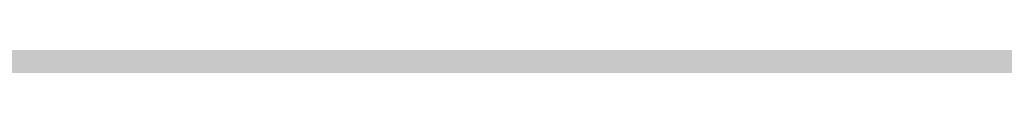
# Model space of a CAD drawing. Units: millimetres. Extents: x 0 to 2267, y 0 to 1823.
# Tile 98 of 256: x 1600.369 to 1605.705, y 1227.263 to 1227.331. Entities that reach past the tile are written whole.
import ezdxf

# ---------------------------------------------------------------- set-up
doc = ezdxf.new("R2010")
doc.units = ezdxf.units.MM
doc.header["$MEASUREMENT"] = 0
doc.layers.add('M-DIMS', color=2, linetype='Continuous', lineweight=25)
doc.layers.add('M-HATC', color=252, linetype='Continuous', lineweight=18)
doc.styles.get("Standard").update_dxf_attribs({"font": 'arial.ttf'})
doc.dimstyles.get("Standard").update_dxf_attribs({"dimtxt": 7, "dimasz": 4, "dimexe": 0.18, "dimexo": 0.0625, "dimgap": 0.09, "dimtad": 0, "dimdec": 0, "dimzin": 0, "dimdsep": 46, "dimtxsty": 'Standard', "dimcen": 0.09, "dimadec": 0, "dimazin": 0, "dimtfac": 1, "dimtdec": 0, "dimtofl": 0, "dimtmove": 0, "dimatfit": 3, "dimfxl": 1, "dimtolj": 1, "dimtzin": 0, "dimarcsym": 0})

# ---------------------------------------------------------------- blocks, each defined once
blk = doc.blocks.new('*D19')
at = {"layer": 'Defpoints', "color": 0, "transparency": 16777216}
for p in [(1605.3399, 1483.3044), (1445.5291, 1333.8851)]:
    blk.add_point(p, dxfattribs=at)
at = {"layer": 'M-DIMS', "color": 0, "lineweight": -2, "transparency": 16777216}
for p, q in [((1605.3399, 1483.2144), (1605.3399, 1483.3944)), ((1605.2499, 1483.3044), (1605.4299, 1483.3044)), ((1366.3244, 1259.8306), (1442.6072, 1331.1532))]:
    blk.add_line(p, q, dxfattribs=at)
at = {"layer": 'M-DIMS', "color": 0, "transparency": 16777216}
blk.add_solid([(1442.1519, 1331.6402), (1443.0625, 1330.6663), (1445.5291, 1333.8851)], dxfattribs=at)
at = {"layer": 'M-DIMS', "color": 0, "transparency": 16777216, "insert": (1349.6425, 1244.2335), "char_height": 7, "attachment_point": 5, "rotation": 43.0753}
blk.add_mtext('\\A1;2X R218.8', dxfattribs=at)

msp = doc.modelspace()

# ---------------------------------------------------------------- hatches: boundary and pattern name
at = {"layer": 'M-HATC'}
h = msp.add_hatch(color=256, dxfattribs=at)
h.dxf.hatch_style = 1
h.paths.add_polyline_path([(2055.771, 1603.062), (1381.0868, 1603.062), (1381.0868, 1598.062), (2055.771, 1598.062)])
h.paths.add_polyline_path([(2055.771, 1598.062), (1381.0868, 1598.062), (1381.0868, 1593.062), (2055.771, 1593.062)])
h.paths.add_polyline_path([(2051.3074, 1536.7609), (1385.5504, 1536.7609), (1385.5504, 1526.7609), (1387.5504, 1526.7609), (1388.5366, 1525.0528), (1385.3319, 1521.2335), (1385.3319, 1521.2226), (2050.2542, 1522.7491), (2048.3212, 1525.0528), (2049.3074, 1526.7609), (2051.3074, 1526.7609)])
edge = h.paths.add_edge_path()
edge.add_arc((1847.5345, 1379.1492), 135, 222.603061, 222.890851, ccw=False)
edge.add_line((1748.1663, 1287.7656), (1683.0921, 1287.7656))
edge.add_arc((1583.7239, 1379.1492), 135, 317.109149, 317.396939, ccw=False)
edge.add_arc((1678.9686, 1290.6707), 5, 222.8909, 317.1091, ccw=False)
edge.add_arc((1774.2133, 1379.1492), 135, 222.603061, 222.890851, ccw=False)
edge.add_line((1674.8451, 1287.7656), (1609.7709, 1287.7656))
edge.add_arc((1510.4027, 1379.1492), 135, 317.109149, 317.396939, ccw=False)
edge.add_arc((1605.6474, 1290.6707), 5, 222.8909, 317.1091, ccw=False)
edge.add_arc((1700.8921, 1379.1492), 135, 222.603061, 222.890851, ccw=False)
edge.add_line((1601.5239, 1287.7656), (1536.4497, 1287.7656))
edge.add_arc((1437.0815, 1379.1492), 135, 317.109149, 317.396939, ccw=False)
edge.add_arc((1532.3262, 1290.6707), 5, 222.8909, 317.1091, ccw=False)
edge.add_arc((1627.5709, 1379.1492), 135, 222.603061, 222.890851, ccw=False)
edge.add_line((1528.2027, 1287.7656), (1505.9289, 1287.7656))
edge.add_spline(control_points=[(1505.9289, 1287.7656), (1504.2622, 1287.7656), (1504.2622, 1282.7656), (1505.9289, 1282.7656)], knot_values=[0, 0, 0, 0, 5, 5, 5, 5], degree=3, periodic=0)
edge.add_line((1505.9289, 1282.7656), (1930.9289, 1282.7656))
edge.add_spline(control_points=[(1930.9289, 1282.7656), (1932.5956, 1282.7656), (1932.5956, 1287.7656), (1930.9289, 1287.7656)], knot_values=[0, 0, 0, 0, 5, 5, 5, 5], degree=3, periodic=0)
edge.add_line((1930.9289, 1287.7656), (1903.0557, 1287.7656))
edge.add_arc((1803.6875, 1379.1492), 135, 317.109149, 317.396939, ccw=False)
edge.add_arc((1898.9322, 1290.6707), 5, 222.8909, 317.1091, ccw=False)
edge.add_arc((1994.1769, 1379.1492), 135, 222.603061, 222.890851, ccw=False)
edge.add_line((1894.8087, 1287.7656), (1829.7345, 1287.7656))
edge.add_arc((1730.3663, 1379.1492), 135, 317.109149, 317.396939, ccw=False)
edge.add_arc((1825.611, 1290.6707), 5, 222.8909, 317.1091, ccw=False)
edge.add_arc((1920.8557, 1379.1492), 135, 222.603061, 222.890851, ccw=False)
edge.add_line((1821.4875, 1287.7656), (1756.4133, 1287.7656))
edge.add_arc((1657.0451, 1379.1492), 135, 317.109149, 317.396939, ccw=False)
edge.add_arc((1752.2898, 1290.6707), 5, 222.8909, 317.1091, ccw=False)
edge = h.paths.add_edge_path()
edge.add_spline(control_points=[(1843.4289, 1227.2475), (1845.0956, 1227.2475), (1845.0956, 1232.2475), (1843.4289, 1232.2475)], knot_values=[0, 0, 0, 0, 5, 5, 5, 5], degree=3, periodic=0)
edge.add_line((1843.4289, 1232.2475), (1593.4289, 1232.2475))
edge.add_spline(control_points=[(1593.4289, 1232.2475), (1591.7622, 1232.2475), (1591.7622, 1227.2475), (1593.4289, 1227.2475)], knot_values=[0, 0, 0, 0, 5, 5, 5, 5], degree=3, periodic=0)
edge.add_line((1593.4289, 1227.2475), (1843.4289, 1227.2475))
h.paths.add_polyline_path([(1905.9289, 1127.4171), (1530.9289, 1127.4171, 0.414214), (1520.9289, 1117.4171), (1530.9289, 1117.4171), (1915.9289, 1117.4171, 0.414214)])
edge = h.paths.add_edge_path()
edge.add_arc((1397.0858, 1498.4078), 12.7299, 90.78215, 190.87871, ccw=False)
edge.add_line((1396.912, 1511.1365), (1428.0097, 1511.3488))
edge.add_line((1428.0097, 1511.3488), (1433.0097, 1511.3488))
edge.add_line((1433.0097, 1511.3488), (1434.439, 1511.3488))
edge.add_arc((1419.474, 1498.0804), 20, 41.561, 74.08211)
edge.add_line((1424.9592, 1517.3135), (1399.9351, 1517.2561))
edge.add_spline(control_points=[(1399.9307, 1517.2561), (1399.884, 1517.2131), (1399.8328, 1517.1689), (1399.7774, 1517.1236)], knot_values=[11.567499, 11.567499, 11.567499, 11.567499, 11.814249, 11.814249, 11.814249, 11.814249], degree=3, periodic=0)
edge.add_spline(control_points=[(1399.6328, 1517.0099), (1399.5831, 1516.9721), (1399.5307, 1516.9338), (1399.4759, 1516.8947)], knot_values=[11.167718, 11.167718, 11.167718, 11.167718, 11.365188, 11.365188, 11.365188, 11.365188], degree=3, periodic=0)
edge.add_spline(control_points=[(1399.3398, 1516.8001), (1399.1514, 1516.6719), (1398.9384, 1516.5377), (1398.704, 1516.3994)], knot_values=[10.376405, 10.376405, 10.376405, 10.376405, 11.00994, 11.00994, 11.00994, 11.00994], degree=3, periodic=0)
edge.add_spline(control_points=[(1398.6572, 1516.3719), (1398.5789, 1516.326), (1398.4983, 1516.2797), (1398.4155, 1516.2331)], knot_values=[10.125175, 10.125175, 10.125175, 10.125175, 10.334406, 10.334406, 10.334406, 10.334406], degree=3, periodic=0)
edge.add_spline(control_points=[(1398.2642, 1516.1487), (1398.196, 1516.1111), (1398.1263, 1516.0732), (1398.0555, 1516.0351)], knot_values=[9.832246, 9.832246, 9.832246, 9.832246, 9.999658, 9.999658, 9.999658, 9.999658], degree=3, periodic=0)
edge.add_spline(control_points=[(1397.9987, 1516.0048), (1397.7312, 1515.8621), (1397.446, 1515.7171), (1397.1466, 1515.5714)], knot_values=[9.161808, 9.161808, 9.161808, 9.161808, 9.787769, 9.787769, 9.787769, 9.787769], degree=3, periodic=0)
edge.add_spline(control_points=[(1397.1466, 1515.5714), (1396.8418, 1515.423), (1396.5222, 1515.274), (1396.1914, 1515.1262)], knot_values=[8.524455, 8.524455, 8.524455, 8.524455, 9.161808, 9.161808, 9.161808, 9.161808], degree=3, periodic=0)
edge.add_spline(control_points=[(1396.0777, 1515.0756), (1395.9854, 1515.0348), (1395.8922, 1514.994), (1395.7983, 1514.9534)], knot_values=[8.275193, 8.275193, 8.275193, 8.275193, 8.451726, 8.451726, 8.451726, 8.451726], degree=3, periodic=0)
edge.add_spline(control_points=[(1395.6018, 1514.8691), (1395.4997, 1514.8257), (1395.3968, 1514.7824), (1395.2932, 1514.7394)], knot_values=[7.962917, 7.962917, 7.962917, 7.962917, 8.152764, 8.152764, 8.152764, 8.152764], degree=3, periodic=0)
edge.add_spline(control_points=[(1395.2116, 1514.7057), (1394.8278, 1514.5475), (1394.4345, 1514.3929), (1394.0364, 1514.2442)], knot_values=[7.21254, 7.21254, 7.21254, 7.21254, 7.913148, 7.913148, 7.913148, 7.913148], degree=3, periodic=0)
edge.add_spline(control_points=[(1394.0364, 1514.2442), (1393.7076, 1514.1214), (1393.3754, 1514.0027), (1393.0427, 1513.8895)], knot_values=[6.633733, 6.633733, 6.633733, 6.633733, 7.21254, 7.21254, 7.21254, 7.21254], degree=3, periodic=0)
edge.add_spline(control_points=[(1392.8214, 1513.815), (1392.7198, 1513.7812), (1392.6181, 1513.7479), (1392.5166, 1513.7152)], knot_values=[6.328796, 6.328796, 6.328796, 6.328796, 6.505493, 6.505493, 6.505493, 6.505493], degree=3, periodic=0)
edge.add_spline(control_points=[(1392.5166, 1513.7152), (1392.3187, 1513.6515), (1392.1212, 1513.59), (1391.9244, 1513.531)], knot_values=[5.984605, 5.984605, 5.984605, 5.984605, 6.328796, 6.328796, 6.328796, 6.328796], degree=3, periodic=0)
edge.add_spline(control_points=[(1391.7915, 1513.4915), (1391.3122, 1513.3501), (1390.8384, 1513.2239), (1390.3784, 1513.1171)], knot_values=[5.066697, 5.066697, 5.066697, 5.066697, 5.907055, 5.907055, 5.907055, 5.907055], degree=3, periodic=0)
edge.add_spline(control_points=[(1390.3784, 1513.1171), (1390.1797, 1513.071), (1389.9836, 1513.0284), (1389.7907, 1512.9899)], knot_values=[4.70367, 4.70367, 4.70367, 4.70367, 5.066695, 5.066695, 5.066695, 5.066695], degree=3, periodic=0)
edge.add_spline(control_points=[(1389.422, 1512.9204), (1389.2459, 1512.8892), (1389.0729, 1512.8617), (1388.9036, 1512.8381)], knot_values=[4.130571, 4.130571, 4.130571, 4.130571, 4.469816, 4.469816, 4.469816, 4.469816], degree=3, periodic=0)
edge.add_spline(control_points=[(1388.9036, 1512.8381), (1388.591, 1512.7946), (1388.2911, 1512.7644), (1388.0071, 1512.7494)], knot_values=[3.504031, 3.504031, 3.504031, 3.504031, 4.130571, 4.130571, 4.130571, 4.130571], degree=3, periodic=0)
edge.add_spline(control_points=[(1387.9356, 1512.7459), (1387.8538, 1512.7423), (1387.7733, 1512.74), (1387.6944, 1512.739)], knot_values=[3.268866, 3.268866, 3.268866, 3.268866, 3.451164, 3.451164, 3.451164, 3.451164], degree=3, periodic=0)
edge.add_spline(control_points=[(1387.3351, 1512.7443), (1387.2076, 1512.7499), (1387.0847, 1512.7597), (1386.967, 1512.7739)], knot_values=[2.670686, 2.670686, 2.670686, 2.670686, 2.984, 2.984, 2.984, 2.984], degree=3, periodic=0)
edge.add_spline(control_points=[(1386.8327, 1512.7922), (1386.8209, 1512.7941), (1386.8092, 1512.7959), (1386.7975, 1512.7979)], knot_values=[2.516981, 2.516981, 2.516981, 2.516981, 2.549528, 2.549528, 2.549528, 2.549528], degree=3, periodic=0)
edge.add_spline(control_points=[(1386.4526, 1512.8735), (1386.4257, 1512.881), (1386.3993, 1512.889), (1386.3733, 1512.8972)], knot_values=[2.095869, 2.095869, 2.095869, 2.095869, 2.17941, 2.17941, 2.17941, 2.17941], degree=3, periodic=0)
edge.add_spline(control_points=[(1386.0691, 1513.0189), (1386.0634, 1513.0217), (1386.0577, 1513.0246), (1386.052, 1513.0275)], knot_values=[1.72453, 1.72453, 1.72453, 1.72453, 1.745933, 1.745933, 1.745933, 1.745933], degree=3, periodic=0)
edge.add_arc((1399.474, 1498.0804), 20, 131.82432, 180)
edge.add_arc((1630.3336, 1505.5484), 250.9708, 181.705176, 236.427975)
edge.add_arc((1605.3399, 1483.3044), 218.7822, 238.660829, 243.34961)
edge.add_arc((1647.0911, 1510.3592), 262.8986, 183.129836, 237.853442, ccw=False)
h.paths.add_polyline_path([(1406.5369, 1391.9644, 0.149382), (1491.5506, 1296.4418, -0.129517)], flags=17)
edge = h.paths.add_edge_path()
edge.add_arc((2037.3838, 1498.0804), 20, 0, 48.26587)
edge.add_spline(control_points=[(2050.6973, 1513.0052), (2050.6512, 1512.9847), (2050.6034, 1512.9655), (2050.5539, 1512.9477)], knot_values=[1.835652, 1.835652, 1.835652, 1.835652, 2.000781, 2.000781, 2.000781, 2.000781], degree=3, periodic=0)
edge.add_spline(control_points=[(2050.4616, 1512.9166), (2050.479, 1512.9221), (2050.4963, 1512.9277), (2050.5133, 1512.9335)], knot_values=[2.045477, 2.045477, 2.045477, 2.045477, 2.101389, 2.101389, 2.101389, 2.101389], degree=3, periodic=0)
edge.add_spline(control_points=[(2050.129, 1512.8342), (2050.1984, 1512.8473), (2050.2657, 1512.8623), (2050.3308, 1512.8792)], knot_values=[2.237629, 2.237629, 2.237629, 2.237629, 2.435841, 2.435841, 2.435841, 2.435841], degree=3, periodic=0)
edge.add_spline(control_points=[(2050.0946, 1512.8278), (2050.1061, 1512.8299), (2050.1176, 1512.832), (2050.129, 1512.8342)], knot_values=[2.435841, 2.435841, 2.435841, 2.435841, 2.468321, 2.468321, 2.468321, 2.468321], degree=3, periodic=0)
edge.add_spline(control_points=[(2049.7843, 1512.7851), (2049.8552, 1512.7922), (2049.9243, 1512.8008), (2049.9917, 1512.8109)], knot_values=[2.563852, 2.563852, 2.563852, 2.563852, 2.748541, 2.748541, 2.748541, 2.748541], degree=3, periodic=0)
edge.add_spline(control_points=[(2049.4052, 1512.7617), (2049.5364, 1512.7653), (2049.6629, 1512.773), (2049.7843, 1512.7851)], knot_values=[2.748541, 2.748541, 2.748541, 2.748541, 3.064882, 3.064882, 3.064882, 3.064882], degree=3, periodic=0)
edge.add_spline(control_points=[(2049.1698, 1512.7597), (2049.2336, 1512.7591), (2049.2965, 1512.7594), (2049.3584, 1512.7606)], knot_values=[3.102309, 3.102309, 3.102309, 3.102309, 3.2503, 3.2503, 3.2503, 3.2503], degree=3, periodic=0)
edge.add_spline(control_points=[(2048.8573, 1512.7691), (2048.9638, 1512.7638), (2049.068, 1512.7606), (2049.1698, 1512.7597)], knot_values=[3.2503, 3.2503, 3.2503, 3.2503, 3.486069, 3.486069, 3.486069, 3.486069], degree=3, periodic=0)
edge.add_spline(control_points=[(2048.6924, 1512.7789), (2048.3729, 1512.8009), (2048.0345, 1512.8411), (2047.6817, 1512.897)], knot_values=[3.606429, 3.606429, 3.606429, 3.606429, 4.2989, 4.2989, 4.2989, 4.2989], degree=3, periodic=0)
edge.add_spline(control_points=[(2047.6817, 1512.897), (2047.5458, 1512.9185), (2047.4077, 1512.9424), (2047.2678, 1512.9685)], knot_values=[4.2989, 4.2989, 4.2989, 4.2989, 4.565769, 4.565769, 4.565769, 4.565769], degree=3, periodic=0)
edge.add_spline(control_points=[(2047.2678, 1512.9685), (2047.1449, 1512.9914), (2047.0207, 1513.016), (2046.8951, 1513.0422)], knot_values=[4.565769, 4.565769, 4.565769, 4.565769, 4.799971, 4.799971, 4.799971, 4.799971], degree=3, periodic=0)
edge.add_spline(control_points=[(2046.8951, 1513.0422), (2046.5286, 1513.1188), (2046.1513, 1513.209), (2045.7676, 1513.3107)], knot_values=[4.799971, 4.799971, 4.799971, 4.799971, 5.483718, 5.483718, 5.483718, 5.483718], degree=3, periodic=0)
edge.add_spline(control_points=[(2045.7676, 1513.3107), (2045.3724, 1513.4154), (2044.9704, 1513.5322), (2044.5662, 1513.6588)], knot_values=[5.483718, 5.483718, 5.483718, 5.483718, 6.187866, 6.187866, 6.187866, 6.187866], degree=3, periodic=0)
edge.add_spline(control_points=[(2044.5662, 1513.6588), (2044.4149, 1513.7061), (2044.2633, 1513.7549), (2044.1116, 1513.8048)], knot_values=[6.187866, 6.187866, 6.187866, 6.187866, 6.451551, 6.451551, 6.451551, 6.451551], degree=3, periodic=0)
edge.add_spline(control_points=[(2044.1116, 1513.8048), (2043.9967, 1513.8427), (2043.8817, 1513.8813), (2043.7668, 1513.9205)], knot_values=[6.451551, 6.451551, 6.451551, 6.451551, 6.651434, 6.651434, 6.651434, 6.651434], degree=3, periodic=0)
edge.add_spline(control_points=[(2043.7668, 1513.9205), (2043.3716, 1514.0554), (2042.9774, 1514.1979), (2042.5886, 1514.3458)], knot_values=[6.651434, 6.651434, 6.651434, 6.651434, 7.338879, 7.338879, 7.338879, 7.338879], degree=3, periodic=0)
edge.add_spline(control_points=[(2042.5886, 1514.3458), (2042.1643, 1514.5071), (2041.7465, 1514.6749), (2041.3409, 1514.846)], knot_values=[7.338879, 7.338879, 7.338879, 7.338879, 8.089209, 8.089209, 8.089209, 8.089209], degree=3, periodic=0)
edge.add_spline(control_points=[(2041.3409, 1514.846), (2041.1028, 1514.9465), (2040.869, 1515.0481), (2040.6405, 1515.1502)], knot_values=[8.089209, 8.089209, 8.089209, 8.089209, 8.529587, 8.529587, 8.529587, 8.529587], degree=3, periodic=0)
edge.add_spline(control_points=[(2040.51, 1515.2089), (2040.0824, 1515.4022), (2039.6747, 1515.5971), (2039.295, 1515.7894)], knot_values=[8.613818, 8.613818, 8.613818, 8.613818, 9.44571, 9.44571, 9.44571, 9.44571], degree=3, periodic=0)
edge.add_spline(control_points=[(2039.295, 1515.7894), (2039.0618, 1515.9075), (2038.8391, 1516.0246), (2038.6288, 1516.1398)], knot_values=[9.44571, 9.44571, 9.44571, 9.44571, 9.956404, 9.956404, 9.956404, 9.956404], degree=3, periodic=0)
edge.add_spline(control_points=[(2038.6288, 1516.1398), (2038.5187, 1516.2001), (2038.4121, 1516.2598), (2038.309, 1516.3189)], knot_values=[9.956404, 9.956404, 9.956404, 9.956404, 10.223542, 10.223542, 10.223542, 10.223542], degree=3, periodic=0)
edge.add_spline(control_points=[(2038.309, 1516.3189), (2038.2138, 1516.3735), (2038.1216, 1516.4276), (2038.0328, 1516.481)], knot_values=[10.223542, 10.223542, 10.223542, 10.223542, 10.47051, 10.47051, 10.47051, 10.47051], degree=3, periodic=0)
edge.add_spline(control_points=[(2038.0328, 1516.481), (2037.7855, 1516.6296), (2037.5639, 1516.773), (2037.3722, 1516.909)], knot_values=[10.47051, 10.47051, 10.47051, 10.47051, 11.15767, 11.15767, 11.15767, 11.15767], degree=3, periodic=0)
edge.add_spline(control_points=[(2037.3722, 1516.909), (2037.2789, 1516.9752), (2037.1927, 1517.0396), (2037.1142, 1517.102)], knot_values=[11.15767, 11.15767, 11.15767, 11.15767, 11.49227, 11.49227, 11.49227, 11.49227], degree=3, periodic=0)
edge.add_spline(control_points=[(2036.8564, 1517.3259), (2036.9148, 1517.2692), (2036.9814, 1517.2103), (2037.0557, 1517.1492)], knot_values=[11.577341, 11.577341, 11.577341, 11.577341, 11.91035, 11.91035, 11.91035, 11.91035], degree=3, periodic=0)
edge.add_spline(control_points=[(2036.8074, 1517.3748), (2036.823, 1517.3587), (2036.8393, 1517.3424), (2036.8564, 1517.3259)], knot_values=[11.91035, 11.91035, 11.91035, 11.91035, 12.007402, 12.007402, 12.007402, 12.007402], degree=3, periodic=0)
edge.add_spline(control_points=[(2036.7017, 1517.494), (2036.7104, 1517.483), (2036.7196, 1517.4719), (2036.7291, 1517.4606)], knot_values=[12.184155, 12.184155, 12.184155, 12.184155, 12.255409, 12.255409, 12.255409, 12.255409], degree=3, periodic=0)
edge.add_spline(control_points=[(2036.6159, 1517.6205), (2036.62, 1517.613), (2036.6243, 1517.6055), (2036.6289, 1517.5979)], knot_values=[12.487913, 12.487913, 12.487913, 12.487913, 12.541035, 12.541035, 12.541035, 12.541035], degree=3, periodic=0)
edge.add_spline(control_points=[(2036.5635, 1517.786), (2036.5637, 1517.7794), (2036.5642, 1517.7726), (2036.565, 1517.7658)], knot_values=[12.911761, 12.911761, 12.911761, 12.911761, 12.968286, 12.968286, 12.968286, 12.968286], degree=3, periodic=0)
edge.add_spline(control_points=[(2036.6166, 1517.9304), (2036.6125, 1517.9259), (2036.6086, 1517.9212), (2036.6049, 1517.9165)], knot_values=[13.382527, 13.382527, 13.382527, 13.382527, 13.433791, 13.433791, 13.433791, 13.433791], degree=3, periodic=0)
edge.add_spline(control_points=[(2036.749, 1518.017), (2036.7361, 1518.0116), (2036.7239, 1518.006), (2036.7124, 1518.0002)], knot_values=[13.726299, 13.726299, 13.726299, 13.726299, 13.809928, 13.809928, 13.809928, 13.809928], degree=3, periodic=0)
edge.add_spline(control_points=[(2036.8604, 1518.0528), (2036.8386, 1518.0474), (2036.8181, 1518.0416), (2036.7988, 1518.0353)], knot_values=[13.910887, 13.910887, 13.910887, 13.910887, 14.02153, 14.02153, 14.02153, 14.02153], degree=3, periodic=0)
edge.add_line((2036.9639, 1518.0804), (2032.3838, 1518.0804))
edge.add_line((2032.3838, 1518.0804), (2027.3838, 1518.0804))
edge.add_line((2027.3838, 1518.0804), (2022.3838, 1518.0804))
edge.add_line((2022.3838, 1518.0804), (2017.3838, 1518.0804))
edge.add_arc((2017.3838, 1498.0804), 20, 90, 138.439)
edge.add_line((2002.4188, 1511.3488), (2003.8481, 1511.3488))
edge.add_line((2003.8481, 1511.3488), (2008.8481, 1511.3488))
edge.add_line((2008.8481, 1511.3488), (2039.772, 1511.1377))
edge.add_arc((2039.772, 1498.4078), 12.7299, -10.87871, 90, ccw=False)
edge.add_arc((1789.7668, 1510.3592), 262.8986, 302.146558, 356.870164, ccw=False)
edge.add_arc((1831.5179, 1483.3044), 218.7822, 296.65039, 301.339171)
edge.add_arc((1806.5242, 1505.5484), 250.9708, 303.572025, 358.294824)
h.paths.add_polyline_path([(2030.321, 1391.9644, -0.129517), (1945.3072, 1296.4418, 0.149382)], flags=17)
edge = h.paths.add_edge_path()
edge.add_spline(control_points=[(2037.2464, 1518.0821), (2037.2898, 1518.081), (2037.3355, 1518.0804), (2037.3838, 1518.0804)], knot_values=[0.000012, 0.000012, 0.000012, 0.000012, 0.144754, 0.144754, 0.144754, 0.144754], degree=3, periodic=0)
edge.add_line((2037.3357, 1518.0804), (2037.0096, 1518.0804))
edge.add_spline(control_points=[(2037.0096, 1518.0804), (2036.9822, 1518.0768), (2036.956, 1518.0727), (2036.9312, 1518.0681)], knot_values=[14.13465, 14.13465, 14.13465, 14.13465, 14.247197, 14.247197, 14.247197, 14.247197], degree=3, periodic=0)
edge.add_spline(control_points=[(2036.9312, 1518.0681), (2036.9276, 1518.0674), (2036.9241, 1518.0667), (2036.9205, 1518.0661)], knot_values=[14.118315, 14.118315, 14.118315, 14.118315, 14.13465, 14.13465, 14.13465, 14.13465], degree=3, periodic=0)
edge.add_spline(control_points=[(2036.9205, 1518.0661), (2036.9118, 1518.0644), (2036.9032, 1518.0626), (2036.8948, 1518.0608)], knot_values=[14.078086, 14.078086, 14.078086, 14.078086, 14.118315, 14.118315, 14.118315, 14.118315], degree=3, periodic=0)
edge.add_spline(control_points=[(2036.8948, 1518.0608), (2036.883, 1518.0583), (2036.8716, 1518.0556), (2036.8604, 1518.0528)], knot_values=[14.02153, 14.02153, 14.02153, 14.02153, 14.078086, 14.078086, 14.078086, 14.078086], degree=3, periodic=0)
edge.add_spline(control_points=[(2036.8604, 1518.0528), (2036.8386, 1518.0474), (2036.8181, 1518.0416), (2036.7988, 1518.0353)], knot_values=[13.910887, 13.910887, 13.910887, 13.910887, 14.02153, 14.02153, 14.02153, 14.02153], degree=3, periodic=0)
edge.add_spline(control_points=[(2036.7988, 1518.0353), (2036.7981, 1518.035), (2036.7974, 1518.0348), (2036.7967, 1518.0346)], knot_values=[13.906906, 13.906906, 13.906906, 13.906906, 13.910887, 13.910887, 13.910887, 13.910887], degree=3, periodic=0)
edge.add_spline(control_points=[(2036.7967, 1518.0346), (2036.7882, 1518.0318), (2036.7799, 1518.0289), (2036.7719, 1518.0259)], knot_values=[13.857826, 13.857826, 13.857826, 13.857826, 13.906906, 13.906906, 13.906906, 13.906906], degree=3, periodic=0)
edge.add_spline(control_points=[(2036.7719, 1518.0259), (2036.764, 1518.023), (2036.7564, 1518.02), (2036.749, 1518.017)], knot_values=[13.809928, 13.809928, 13.809928, 13.809928, 13.857826, 13.857826, 13.857826, 13.857826], degree=3, periodic=0)
edge.add_spline(control_points=[(2036.749, 1518.017), (2036.7361, 1518.0116), (2036.7239, 1518.006), (2036.7124, 1518.0002)], knot_values=[13.726299, 13.726299, 13.726299, 13.726299, 13.809928, 13.809928, 13.809928, 13.809928], degree=3, periodic=0)
edge.add_spline(control_points=[(2036.7124, 1518.0002), (2036.7121, 1518), (2036.7118, 1517.9999), (2036.7115, 1517.9997)], knot_values=[13.723993, 13.723993, 13.723993, 13.723993, 13.726299, 13.726299, 13.726299, 13.726299], degree=3, periodic=0)
edge.add_spline(control_points=[(2036.7115, 1517.9997), (2036.7063, 1517.9971), (2036.7013, 1517.9944), (2036.6965, 1517.9917)], knot_values=[13.686536, 13.686536, 13.686536, 13.686536, 13.723993, 13.723993, 13.723993, 13.723993], degree=3, periodic=0)
edge.add_spline(control_points=[(2036.6965, 1517.9917), (2036.6919, 1517.9891), (2036.6874, 1517.9865), (2036.6831, 1517.9839)], knot_values=[13.651251, 13.651251, 13.651251, 13.651251, 13.686536, 13.686536, 13.686536, 13.686536], degree=3, periodic=0)
edge.add_spline(control_points=[(2036.6831, 1517.9839), (2036.6764, 1517.9798), (2036.67, 1517.9757), (2036.6639, 1517.9714)], knot_values=[13.596804, 13.596804, 13.596804, 13.596804, 13.651251, 13.651251, 13.651251, 13.651251], degree=3, periodic=0)
edge.add_spline(control_points=[(2036.6639, 1517.9714), (2036.6636, 1517.9712), (2036.6633, 1517.9709), (2036.6629, 1517.9707)], knot_values=[13.593956, 13.593956, 13.593956, 13.593956, 13.596804, 13.596804, 13.596804, 13.596804], degree=3, periodic=0)
edge.add_spline(control_points=[(2036.6629, 1517.9707), (2036.6603, 1517.9689), (2036.6577, 1517.967), (2036.6552, 1517.9651)], knot_values=[13.570322, 13.570322, 13.570322, 13.570322, 13.593956, 13.593956, 13.593956, 13.593956], degree=3, periodic=0)
edge.add_spline(control_points=[(2036.6552, 1517.9651), (2036.6525, 1517.9631), (2036.6499, 1517.9611), (2036.6474, 1517.9591)], knot_values=[13.545477, 13.545477, 13.545477, 13.545477, 13.570322, 13.570322, 13.570322, 13.570322], degree=3, periodic=0)
edge.add_spline(control_points=[(2036.6474, 1517.9591), (2036.6472, 1517.9589), (2036.6471, 1517.9588), (2036.6469, 1517.9587)], knot_values=[13.543931, 13.543931, 13.543931, 13.543931, 13.545477, 13.545477, 13.545477, 13.545477], degree=3, periodic=0)
edge.add_spline(control_points=[(2036.6469, 1517.9587), (2036.6412, 1517.9541), (2036.6358, 1517.9494), (2036.6307, 1517.9447)], knot_values=[13.488237, 13.488237, 13.488237, 13.488237, 13.543931, 13.543931, 13.543931, 13.543931], degree=3, periodic=0)
edge.add_spline(control_points=[(2036.6307, 1517.9447), (2036.6282, 1517.9423), (2036.6257, 1517.9399), (2036.6233, 1517.9374)], knot_values=[13.460307, 13.460307, 13.460307, 13.460307, 13.488237, 13.488237, 13.488237, 13.488237], degree=3, periodic=0)
edge.add_spline(control_points=[(2036.6233, 1517.9374), (2036.6215, 1517.9356), (2036.6198, 1517.9338), (2036.6181, 1517.932)], knot_values=[13.439712, 13.439712, 13.439712, 13.439712, 13.460307, 13.460307, 13.460307, 13.460307], degree=3, periodic=0)
edge.add_spline(control_points=[(2036.6181, 1517.932), (2036.6176, 1517.9315), (2036.6171, 1517.9309), (2036.6166, 1517.9304)], knot_values=[13.433791, 13.433791, 13.433791, 13.433791, 13.439712, 13.439712, 13.439712, 13.439712], degree=3, periodic=0)
edge.add_spline(control_points=[(2036.6166, 1517.9304), (2036.6125, 1517.9259), (2036.6086, 1517.9212), (2036.6049, 1517.9165)], knot_values=[13.382527, 13.382527, 13.382527, 13.382527, 13.433791, 13.433791, 13.433791, 13.433791], degree=3, periodic=0)
edge.add_spline(control_points=[(2036.6049, 1517.9165), (2036.6026, 1517.9135), (2036.6004, 1517.9104), (2036.5982, 1517.9074)], knot_values=[13.350017, 13.350017, 13.350017, 13.350017, 13.382527, 13.382527, 13.382527, 13.382527], degree=3, periodic=0)
edge.add_spline(control_points=[(2036.5982, 1517.9074), (2036.5972, 1517.9059), (2036.5962, 1517.9043), (2036.5952, 1517.9028)], knot_values=[13.333922, 13.333922, 13.333922, 13.333922, 13.350017, 13.350017, 13.350017, 13.350017], degree=3, periodic=0)
edge.add_spline(control_points=[(2036.5952, 1517.9028), (2036.5945, 1517.9018), (2036.5939, 1517.9009), (2036.5933, 1517.8999)], knot_values=[13.323828, 13.323828, 13.323828, 13.323828, 13.333922, 13.333922, 13.333922, 13.333922], degree=3, periodic=0)
edge.add_spline(control_points=[(2036.5933, 1517.8999), (2036.5905, 1517.8955), (2036.5879, 1517.8909), (2036.5855, 1517.8864)], knot_values=[13.277545, 13.277545, 13.277545, 13.277545, 13.323828, 13.323828, 13.323828, 13.323828], degree=3, periodic=0)
edge.add_spline(control_points=[(2036.5855, 1517.8864), (2036.5836, 1517.8827), (2036.5817, 1517.8789), (2036.5801, 1517.8751)], knot_values=[13.240119, 13.240119, 13.240119, 13.240119, 13.277545, 13.277545, 13.277545, 13.277545], degree=3, periodic=0)
edge.add_spline(control_points=[(2036.5801, 1517.8751), (2036.5795, 1517.8739), (2036.579, 1517.8727), (2036.5785, 1517.8715)], knot_values=[13.228211, 13.228211, 13.228211, 13.228211, 13.240119, 13.240119, 13.240119, 13.240119], degree=3, periodic=0)
edge.add_spline(control_points=[(2036.5785, 1517.8715), (2036.578, 1517.8702), (2036.5774, 1517.869), (2036.5769, 1517.8677)], knot_values=[13.215717, 13.215717, 13.215717, 13.215717, 13.228211, 13.228211, 13.228211, 13.228211], degree=3, periodic=0)
edge.add_spline(control_points=[(2036.5769, 1517.8677), (2036.5755, 1517.864), (2036.5741, 1517.8603), (2036.5729, 1517.8565)], knot_values=[13.179847, 13.179847, 13.179847, 13.179847, 13.215717, 13.215717, 13.215717, 13.215717], degree=3, periodic=0)
edge.add_spline(control_points=[(2036.5729, 1517.8565), (2036.5713, 1517.8515), (2036.5699, 1517.8464), (2036.5687, 1517.8413)], knot_values=[13.132017, 13.132017, 13.132017, 13.132017, 13.179847, 13.179847, 13.179847, 13.179847], degree=3, periodic=0)
edge.add_spline(control_points=[(2036.5687, 1517.8413), (2036.5684, 1517.8402), (2036.5682, 1517.8392), (2036.568, 1517.8382)], knot_values=[13.122482, 13.122482, 13.122482, 13.122482, 13.132017, 13.132017, 13.132017, 13.132017], degree=3, periodic=0)
edge.add_spline(control_points=[(2036.568, 1517.8382), (2036.5676, 1517.8363), (2036.5672, 1517.8345), (2036.5669, 1517.8327)], knot_values=[13.105592, 13.105592, 13.105592, 13.105592, 13.122482, 13.122482, 13.122482, 13.122482], degree=3, periodic=0)
edge.add_spline(control_points=[(2036.5669, 1517.8327), (2036.5662, 1517.8292), (2036.5657, 1517.8257), (2036.5652, 1517.8222)], knot_values=[13.074063, 13.074063, 13.074063, 13.074063, 13.105592, 13.105592, 13.105592, 13.105592], degree=3, periodic=0)
edge.add_spline(control_points=[(2036.5652, 1517.8222), (2036.5652, 1517.8222), (2036.5652, 1517.8222), (2036.5652, 1517.8222)], knot_values=[13.074043, 13.074043, 13.074043, 13.074043, 13.074063, 13.074063, 13.074063, 13.074063], degree=3, periodic=0)
edge.add_spline(control_points=[(2036.5652, 1517.8222), (2036.5644, 1517.8164), (2036.5639, 1517.8106), (2036.5636, 1517.8046)], knot_values=[13.021884, 13.021884, 13.021884, 13.021884, 13.074043, 13.074043, 13.074043, 13.074043], degree=3, periodic=0)
edge.add_spline(control_points=[(2036.5636, 1517.8046), (2036.5636, 1517.804), (2036.5636, 1517.8034), (2036.5635, 1517.8028)], knot_values=[13.01674, 13.01674, 13.01674, 13.01674, 13.021884, 13.021884, 13.021884, 13.021884], degree=3, periodic=0)
edge.add_spline(control_points=[(2036.5635, 1517.8028), (2036.5634, 1517.8005), (2036.5634, 1517.7982), (2036.5634, 1517.7958)], knot_values=[12.996438, 12.996438, 12.996438, 12.996438, 13.01674, 13.01674, 13.01674, 13.01674], degree=3, periodic=0)
edge.add_spline(control_points=[(2036.5634, 1517.7958), (2036.5633, 1517.7926), (2036.5634, 1517.7893), (2036.5635, 1517.786)], knot_values=[12.968286, 12.968286, 12.968286, 12.968286, 12.996438, 12.996438, 12.996438, 12.996438], degree=3, periodic=0)
edge.add_spline(control_points=[(2036.5635, 1517.786), (2036.5637, 1517.7794), (2036.5642, 1517.7726), (2036.565, 1517.7658)], knot_values=[12.911761, 12.911761, 12.911761, 12.911761, 12.968286, 12.968286, 12.968286, 12.968286], degree=3, periodic=0)
edge.add_spline(control_points=[(2036.565, 1517.7658), (2036.565, 1517.7657), (2036.565, 1517.7656), (2036.565, 1517.7656)], knot_values=[12.911017, 12.911017, 12.911017, 12.911017, 12.911761, 12.911761, 12.911761, 12.911761], degree=3, periodic=0)
edge.add_spline(control_points=[(2036.565, 1517.7656), (2036.5654, 1517.7625), (2036.5658, 1517.7593), (2036.5663, 1517.7562)], knot_values=[12.88528, 12.88528, 12.88528, 12.88528, 12.911017, 12.911017, 12.911017, 12.911017], degree=3, periodic=0)
edge.add_spline(control_points=[(2036.5663, 1517.7562), (2036.5667, 1517.7534), (2036.5672, 1517.7506), (2036.5677, 1517.7478)], knot_values=[12.862519, 12.862519, 12.862519, 12.862519, 12.88528, 12.88528, 12.88528, 12.88528], degree=3, periodic=0)
edge.add_spline(control_points=[(2036.5677, 1517.7478), (2036.5678, 1517.7474), (2036.5679, 1517.7469), (2036.568, 1517.7465)], knot_values=[12.858885, 12.858885, 12.858885, 12.858885, 12.862519, 12.862519, 12.862519, 12.862519], degree=3, periodic=0)
edge.add_spline(control_points=[(2036.568, 1517.7465), (2036.5692, 1517.7399), (2036.5707, 1517.7332), (2036.5724, 1517.7264)], knot_values=[12.8053, 12.8053, 12.8053, 12.8053, 12.858885, 12.858885, 12.858885, 12.858885], degree=3, periodic=0)
edge.add_spline(control_points=[(2036.5724, 1517.7264), (2036.5734, 1517.7226), (2036.5745, 1517.7187), (2036.5756, 1517.7149)], knot_values=[12.775176, 12.775176, 12.775176, 12.775176, 12.8053, 12.8053, 12.8053, 12.8053], degree=3, periodic=0)
edge.add_spline(control_points=[(2036.5756, 1517.7149), (2036.5763, 1517.7125), (2036.577, 1517.7102), (2036.5778, 1517.7078)], knot_values=[12.756759, 12.756759, 12.756759, 12.756759, 12.775176, 12.775176, 12.775176, 12.775176], degree=3, periodic=0)
edge.add_spline(control_points=[(2036.5778, 1517.7078), (2036.5781, 1517.7067), (2036.5784, 1517.7057), (2036.5787, 1517.7047)], knot_values=[12.748742, 12.748742, 12.748742, 12.748742, 12.756759, 12.756759, 12.756759, 12.756759], degree=3, periodic=0)
edge.add_spline(control_points=[(2036.5787, 1517.7047), (2036.5808, 1517.6983), (2036.5831, 1517.6919), (2036.5856, 1517.6854)], knot_values=[12.69959, 12.69959, 12.69959, 12.69959, 12.748742, 12.748742, 12.748742, 12.748742], degree=3, periodic=0)
edge.add_spline(control_points=[(2036.5856, 1517.6854), (2036.5876, 1517.68), (2036.5898, 1517.6746), (2036.5921, 1517.6692)], knot_values=[12.659038, 12.659038, 12.659038, 12.659038, 12.69959, 12.69959, 12.69959, 12.69959], degree=3, periodic=0)
edge.add_spline(control_points=[(2036.5921, 1517.6692), (2036.594, 1517.6648), (2036.5959, 1517.6605), (2036.5979, 1517.6561)], knot_values=[12.626806, 12.626806, 12.626806, 12.626806, 12.659038, 12.659038, 12.659038, 12.659038], degree=3, periodic=0)
edge.add_spline(control_points=[(2036.5979, 1517.6561), (2036.5984, 1517.6551), (2036.5989, 1517.6541), (2036.5993, 1517.6531)], knot_values=[12.619394, 12.619394, 12.619394, 12.619394, 12.626806, 12.626806, 12.626806, 12.626806], degree=3, periodic=0)
edge.add_spline(control_points=[(2036.5993, 1517.6531), (2036.6043, 1517.6424), (2036.6099, 1517.6315), (2036.6159, 1517.6205)], knot_values=[12.541039, 12.541039, 12.541039, 12.541039, 12.619394, 12.619394, 12.619394, 12.619394], degree=3, periodic=0)
edge.add_spline(control_points=[(2036.6159, 1517.6205), (2036.6159, 1517.6205), (2036.6159, 1517.6205), (2036.6159, 1517.6205)], knot_values=[12.541035, 12.541035, 12.541035, 12.541035, 12.541039, 12.541039, 12.541039, 12.541039], degree=3, periodic=0)
edge.add_spline(control_points=[(2036.6159, 1517.6205), (2036.62, 1517.613), (2036.6243, 1517.6055), (2036.6289, 1517.5979)], knot_values=[12.487913, 12.487913, 12.487913, 12.487913, 12.541035, 12.541035, 12.541035, 12.541035], degree=3, periodic=0)
edge.add_spline(control_points=[(2036.6289, 1517.5979), (2036.6326, 1517.5916), (2036.6365, 1517.5853), (2036.6406, 1517.5789)], knot_values=[12.443982, 12.443982, 12.443982, 12.443982, 12.487913, 12.487913, 12.487913, 12.487913], degree=3, periodic=0)
edge.add_spline(control_points=[(2036.6406, 1517.5789), (2036.6414, 1517.5776), (2036.6423, 1517.5763), (2036.6431, 1517.5749)], knot_values=[12.434996, 12.434996, 12.434996, 12.434996, 12.443982, 12.443982, 12.443982, 12.443982], degree=3, periodic=0)
edge.add_spline(control_points=[(2036.6431, 1517.5749), (2036.6531, 1517.5596), (2036.6639, 1517.5439), (2036.6756, 1517.528)], knot_values=[12.329647, 12.329647, 12.329647, 12.329647, 12.434996, 12.434996, 12.434996, 12.434996], degree=3, periodic=0)
edge.add_spline(control_points=[(2036.6756, 1517.528), (2036.6839, 1517.5168), (2036.6925, 1517.5055), (2036.7017, 1517.494)], knot_values=[12.255409, 12.255409, 12.255409, 12.255409, 12.329647, 12.329647, 12.329647, 12.329647], degree=3, periodic=0)
edge.add_spline(control_points=[(2036.7017, 1517.494), (2036.7104, 1517.483), (2036.7196, 1517.4719), (2036.7291, 1517.4606)], knot_values=[12.184155, 12.184155, 12.184155, 12.184155, 12.255409, 12.255409, 12.255409, 12.255409], degree=3, periodic=0)
edge.add_spline(control_points=[(2036.7291, 1517.4606), (2036.7436, 1517.4435), (2036.759, 1517.4262), (2036.7753, 1517.4085)], knot_values=[12.075961, 12.075961, 12.075961, 12.075961, 12.184155, 12.184155, 12.184155, 12.184155], degree=3, periodic=0)
edge.add_spline(control_points=[(2036.7753, 1517.4085), (2036.7763, 1517.4075), (2036.7773, 1517.4064), (2036.7783, 1517.4054)], knot_values=[12.069502, 12.069502, 12.069502, 12.069502, 12.075961, 12.075961, 12.075961, 12.075961], degree=3, periodic=0)
edge.add_spline(control_points=[(2036.7783, 1517.4054), (2036.7877, 1517.3953), (2036.7974, 1517.385), (2036.8074, 1517.3748)], knot_values=[12.007402, 12.007402, 12.007402, 12.007402, 12.069502, 12.069502, 12.069502, 12.069502], degree=3, periodic=0)
edge.add_spline(control_points=[(2036.8074, 1517.3748), (2036.823, 1517.3587), (2036.8393, 1517.3424), (2036.8564, 1517.3259)], knot_values=[11.91035, 11.91035, 11.91035, 11.91035, 12.007402, 12.007402, 12.007402, 12.007402], degree=3, periodic=0)
edge.add_spline(control_points=[(2036.8564, 1517.3259), (2036.9148, 1517.2692), (2036.9814, 1517.2103), (2037.0557, 1517.1492)], knot_values=[11.577341, 11.577341, 11.577341, 11.577341, 11.91035, 11.91035, 11.91035, 11.91035], degree=3, periodic=0)
edge.add_spline(control_points=[(2037.0557, 1517.1492), (2037.0747, 1517.1336), (2037.0942, 1517.1179), (2037.1142, 1517.102)], knot_values=[11.49227, 11.49227, 11.49227, 11.49227, 11.577341, 11.577341, 11.577341, 11.577341], degree=3, periodic=0)
edge.add_spline(control_points=[(2037.1142, 1517.102), (2037.1927, 1517.0396), (2037.2789, 1516.9752), (2037.3722, 1516.909)], knot_values=[11.15767, 11.15767, 11.15767, 11.15767, 11.49227, 11.49227, 11.49227, 11.49227], degree=3, periodic=0)
edge.add_spline(control_points=[(2037.3722, 1516.909), (2037.5639, 1516.773), (2037.7855, 1516.6296), (2038.0328, 1516.481)], knot_values=[10.47051, 10.47051, 10.47051, 10.47051, 11.15767, 11.15767, 11.15767, 11.15767], degree=3, periodic=0)
edge.add_spline(control_points=[(2038.0328, 1516.481), (2038.1216, 1516.4276), (2038.2138, 1516.3735), (2038.309, 1516.3189)], knot_values=[10.223542, 10.223542, 10.223542, 10.223542, 10.47051, 10.47051, 10.47051, 10.47051], degree=3, periodic=0)
edge.add_spline(control_points=[(2038.309, 1516.3189), (2038.4121, 1516.2598), (2038.5187, 1516.2001), (2038.6288, 1516.1398)], knot_values=[9.956404, 9.956404, 9.956404, 9.956404, 10.223542, 10.223542, 10.223542, 10.223542], degree=3, periodic=0)
edge.add_spline(control_points=[(2038.6288, 1516.1398), (2038.8391, 1516.0246), (2039.0618, 1515.9075), (2039.295, 1515.7894)], knot_values=[9.44571, 9.44571, 9.44571, 9.44571, 9.956404, 9.956404, 9.956404, 9.956404], degree=3, periodic=0)
edge.add_spline(control_points=[(2039.295, 1515.7894), (2039.6747, 1515.5971), (2040.0824, 1515.4022), (2040.51, 1515.2089)], knot_values=[8.613818, 8.613818, 8.613818, 8.613818, 9.44571, 9.44571, 9.44571, 9.44571], degree=3, periodic=0)
edge.add_spline(control_points=[(2040.51, 1515.2089), (2040.5533, 1515.1893), (2040.5968, 1515.1697), (2040.6405, 1515.1502)], knot_values=[8.529587, 8.529587, 8.529587, 8.529587, 8.613818, 8.613818, 8.613818, 8.613818], degree=3, periodic=0)
edge.add_spline(control_points=[(2040.6405, 1515.1502), (2040.869, 1515.0481), (2041.1028, 1514.9465), (2041.3409, 1514.846)], knot_values=[8.089209, 8.089209, 8.089209, 8.089209, 8.529587, 8.529587, 8.529587, 8.529587], degree=3, periodic=0)
edge.add_spline(control_points=[(2041.3409, 1514.846), (2041.7465, 1514.6749), (2042.1643, 1514.5071), (2042.5886, 1514.3458)], knot_values=[7.338879, 7.338879, 7.338879, 7.338879, 8.089209, 8.089209, 8.089209, 8.089209], degree=3, periodic=0)
edge.add_spline(control_points=[(2042.5886, 1514.3458), (2042.9774, 1514.1979), (2043.3716, 1514.0554), (2043.7668, 1513.9205)], knot_values=[6.651434, 6.651434, 6.651434, 6.651434, 7.338879, 7.338879, 7.338879, 7.338879], degree=3, periodic=0)
edge.add_spline(control_points=[(2043.7668, 1513.9205), (2043.8817, 1513.8813), (2043.9967, 1513.8427), (2044.1116, 1513.8048)], knot_values=[6.451551, 6.451551, 6.451551, 6.451551, 6.651434, 6.651434, 6.651434, 6.651434], degree=3, periodic=0)
edge.add_spline(control_points=[(2044.1116, 1513.8048), (2044.2633, 1513.7549), (2044.4149, 1513.7061), (2044.5662, 1513.6588)], knot_values=[6.187866, 6.187866, 6.187866, 6.187866, 6.451551, 6.451551, 6.451551, 6.451551], degree=3, periodic=0)
edge.add_spline(control_points=[(2044.5662, 1513.6588), (2044.9704, 1513.5322), (2045.3724, 1513.4154), (2045.7676, 1513.3107)], knot_values=[5.483718, 5.483718, 5.483718, 5.483718, 6.187866, 6.187866, 6.187866, 6.187866], degree=3, periodic=0)
edge.add_spline(control_points=[(2045.7676, 1513.3107), (2046.1513, 1513.209), (2046.5286, 1513.1188), (2046.8951, 1513.0422)], knot_values=[4.799971, 4.799971, 4.799971, 4.799971, 5.483718, 5.483718, 5.483718, 5.483718], degree=3, periodic=0)
edge.add_spline(control_points=[(2046.8951, 1513.0422), (2047.0207, 1513.016), (2047.1449, 1512.9914), (2047.2678, 1512.9685)], knot_values=[4.565769, 4.565769, 4.565769, 4.565769, 4.799971, 4.799971, 4.799971, 4.799971], degree=3, periodic=0)
edge.add_spline(control_points=[(2047.2678, 1512.9685), (2047.4077, 1512.9424), (2047.5458, 1512.9185), (2047.6817, 1512.897)], knot_values=[4.2989, 4.2989, 4.2989, 4.2989, 4.565769, 4.565769, 4.565769, 4.565769], degree=3, periodic=0)
edge.add_spline(control_points=[(2047.6817, 1512.897), (2048.0345, 1512.8411), (2048.3729, 1512.8009), (2048.6924, 1512.7789)], knot_values=[3.606429, 3.606429, 3.606429, 3.606429, 4.2989, 4.2989, 4.2989, 4.2989], degree=3, periodic=0)
edge.add_spline(control_points=[(2048.6924, 1512.7789), (2048.7479, 1512.7751), (2048.8029, 1512.7718), (2048.8573, 1512.7691)], knot_values=[3.486069, 3.486069, 3.486069, 3.486069, 3.606429, 3.606429, 3.606429, 3.606429], degree=3, periodic=0)
edge.add_spline(control_points=[(2048.8573, 1512.7691), (2048.9638, 1512.7638), (2049.068, 1512.7606), (2049.1698, 1512.7597)], knot_values=[3.2503, 3.2503, 3.2503, 3.2503, 3.486069, 3.486069, 3.486069, 3.486069], degree=3, periodic=0)
edge.add_spline(control_points=[(2049.1698, 1512.7597), (2049.2336, 1512.7591), (2049.2965, 1512.7594), (2049.3584, 1512.7606)], knot_values=[3.102309, 3.102309, 3.102309, 3.102309, 3.2503, 3.2503, 3.2503, 3.2503], degree=3, periodic=0)
edge.add_spline(control_points=[(2049.3584, 1512.7606), (2049.3741, 1512.7609), (2049.3897, 1512.7613), (2049.4052, 1512.7617)], knot_values=[3.064882, 3.064882, 3.064882, 3.064882, 3.102309, 3.102309, 3.102309, 3.102309], degree=3, periodic=0)
edge.add_spline(control_points=[(2049.4052, 1512.7617), (2049.5364, 1512.7653), (2049.6629, 1512.773), (2049.7843, 1512.7851)], knot_values=[2.748541, 2.748541, 2.748541, 2.748541, 3.064882, 3.064882, 3.064882, 3.064882], degree=3, periodic=0)
edge.add_spline(control_points=[(2049.7843, 1512.7851), (2049.8552, 1512.7922), (2049.9243, 1512.8008), (2049.9917, 1512.8109)], knot_values=[2.563852, 2.563852, 2.563852, 2.563852, 2.748541, 2.748541, 2.748541, 2.748541], degree=3, periodic=0)
edge.add_spline(control_points=[(2049.9917, 1512.8109), (2050.0265, 1512.8161), (2050.0608, 1512.8218), (2050.0946, 1512.8278)], knot_values=[2.468321, 2.468321, 2.468321, 2.468321, 2.563852, 2.563852, 2.563852, 2.563852], degree=3, periodic=0)
edge.add_spline(control_points=[(2050.0946, 1512.8278), (2050.1061, 1512.8299), (2050.1176, 1512.832), (2050.129, 1512.8342)], knot_values=[2.435841, 2.435841, 2.435841, 2.435841, 2.468321, 2.468321, 2.468321, 2.468321], degree=3, periodic=0)
edge.add_spline(control_points=[(2050.129, 1512.8342), (2050.1984, 1512.8473), (2050.2657, 1512.8623), (2050.3308, 1512.8792)], knot_values=[2.237629, 2.237629, 2.237629, 2.237629, 2.435841, 2.435841, 2.435841, 2.435841], degree=3, periodic=0)
edge.add_spline(control_points=[(2050.3308, 1512.8792), (2050.3754, 1512.8908), (2050.4191, 1512.9032), (2050.4616, 1512.9166)], knot_values=[2.101389, 2.101389, 2.101389, 2.101389, 2.237629, 2.237629, 2.237629, 2.237629], degree=3, periodic=0)
edge.add_spline(control_points=[(2050.4616, 1512.9166), (2050.479, 1512.9221), (2050.4963, 1512.9277), (2050.5133, 1512.9335)], knot_values=[2.045477, 2.045477, 2.045477, 2.045477, 2.101389, 2.101389, 2.101389, 2.101389], degree=3, periodic=0)
edge.add_spline(control_points=[(2050.5133, 1512.9335), (2050.527, 1512.9382), (2050.5405, 1512.9429), (2050.5539, 1512.9477)], knot_values=[2.000781, 2.000781, 2.000781, 2.000781, 2.045477, 2.045477, 2.045477, 2.045477], degree=3, periodic=0)
edge.add_spline(control_points=[(2050.5539, 1512.9477), (2050.6034, 1512.9655), (2050.6512, 1512.9847), (2050.6973, 1513.0052)], knot_values=[1.835652, 1.835652, 1.835652, 1.835652, 2.000781, 2.000781, 2.000781, 2.000781], degree=3, periodic=0)
edge.add_arc((2037.3838, 1498.0804), 20, 48.26587, 90.12993)
edge = h.paths.add_edge_path(flags=16)
edge.add_spline(control_points=[(1386.1389, 1512.9859), (1388.92, 1511.7395), (1398.0387, 1515.5187), (1399.9307, 1517.2561)], knot_values=[1.831046, 1.831046, 1.831046, 1.831046, 11.814249, 11.814249, 11.814249, 11.814249], degree=3, periodic=0)
edge.add_line((1399.9307, 1517.2561), (1393.7435, 1517.2419))
edge.add_arc((1399.474, 1498.0804), 20, 106.6501, 131.8173)

# ---------------------------------------------------------------- dimensions: what is measured, and where the dimension line sits
at = {"layer": 'M-DIMS'}
dim = msp.add_radius_dim(center=(1605.3399, 1483.3044), mpoint=(1445.5291, 1333.8851), text='2X <>', dimstyle='Standard', override={"dimdec": 1, "dimlfac": 1, "dimrnd": 0, "dimzin": 0, "dimdsep": 46, "dimlunit": 2}, dxfattribs=at)
dim.commit()
dim.dimension.update_dxf_attribs({"geometry": '*D19', "text_midpoint": (1349.6425, 1244.2335), "dimtype": 164})

doc.saveas('drawing.dxf')
